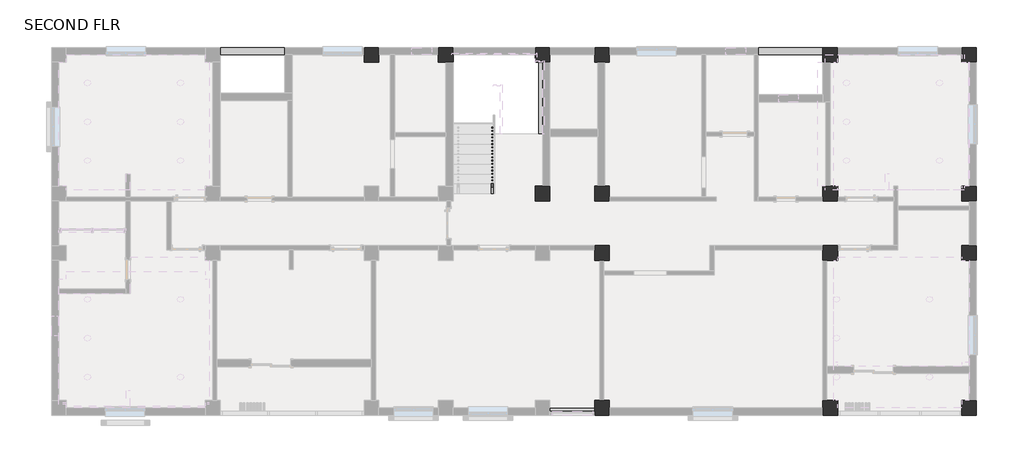
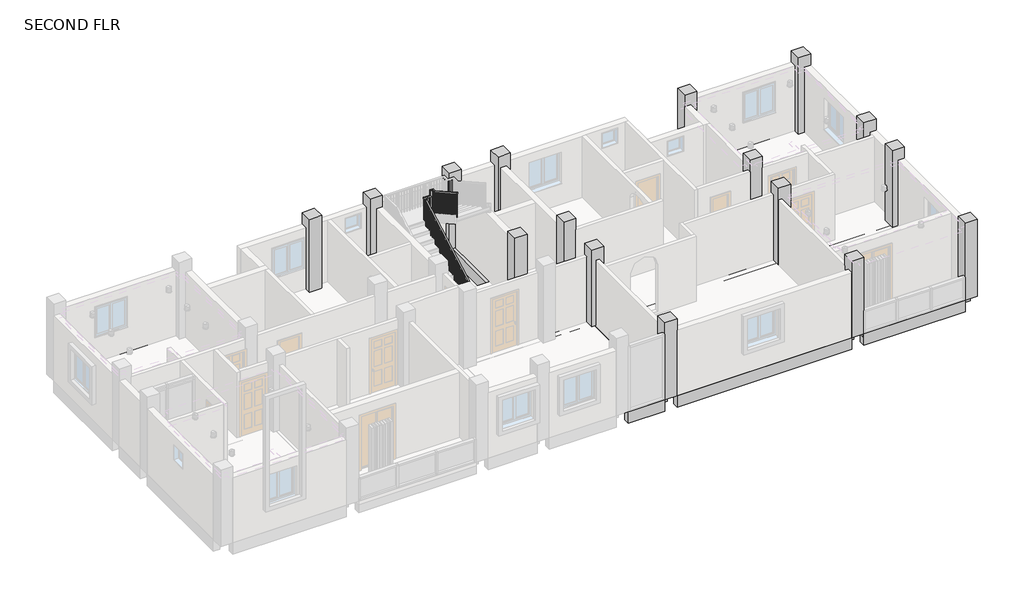
# One storey, part 4 of 5: 29 beams, 16 columns, 1 railing.
"""IFC4 building model written with IfcOpenShell, lengths in millimetres."""

from ifc_helpers import new_model, si_unit, frame, origin, place, context, project, spatial, polyline, outline, extrude, faceted_brep, element, save

model = new_model("IFC4")

# Units and contexts
model_context = context("Model", 3, world=origin())
ifc_project = project(units=[si_unit("LENGTHUNIT", "METRE", prefix="MILLI")], contexts=[model_context])

# Site, building, storey
site = spatial("IfcSite", under=ifc_project)
building = spatial("IfcBuilding", under=site)
storey = spatial("IfcBuildingStorey", under=building, Name="SECOND FLR", Elevation=6400.8)

# Beams
placement = place(None, origin())
element("IfcBeam", 1, ObjectType="Concrete-Rectangular Beam : 9\" X 18\" BEAM", at=placement, inside=storey, context=model_context, shape_type="SweptSolid", body=[
    extrude(outline(polyline([(1310.3916602, -10887.8679047), (1310.3916602, -11116.4679047), (-61.2083398, -11116.4679047), (-61.2083398, -10887.8679047), (1310.3916602, -10887.8679047)])), frame((0.0, 0.0, 5943.6), z_axis=(0.0, 0.0, 1.0), x_axis=(1.0, 0.0, 0.0)), (0.0, 0.0, 1.0), 457.2),
])
element("IfcBeam", 2, ObjectType="Concrete-Rectangular Beam : 9\" X 18\" BEAM", at=placement, inside=storey, context=model_context, shape_type="SweptSolid", body=[
    extrude(outline(polyline([(1424.6916602, -6358.3794704), (1653.2916602, -6358.3794704), (1653.2916602, -10659.2679047), (1424.6916602, -10659.2679047), (1424.6916602, -6358.3794704)])), frame((0.0, 0.0, 5943.6), z_axis=(0.0, 0.0, 1.0), x_axis=(1.0, 0.0, 0.0)), (0.0, 0.0, 1.0), 457.2),
])
element("IfcBeam", 3, ObjectType="Concrete-Rectangular Beam : 9\" X 18\" BEAM", at=placement, inside=storey, context=model_context, shape_type="SweptSolid", body=[
    extrude(outline(polyline([(1424.6916602, -4529.5794704), (1653.2916602, -4529.5794704), (1653.2916602, -5901.1794704), (1424.6916602, -5901.1794704), (1424.6916602, -4529.5794704)])), frame((0.0, 0.0, 5943.6), z_axis=(0.0, 0.0, 1.0), x_axis=(1.0, 0.0, 0.0)), (0.0, 0.0, 1.0), 457.2),
])
element("IfcBeam", 4, ObjectType="Concrete-Rectangular Beam : 9\" X 18\" BEAM", at=placement, inside=storey, context=model_context, shape_type="SweptSolid", body=[
    extrude(outline(polyline([(8317.2128058, -10887.8679047), (8317.2128058, -11116.4679047), (1767.5916602, -11116.4679047), (1767.5916602, -10887.8679047), (8317.2128058, -10887.8679047)])), frame((0.0, 0.0, 5943.6), z_axis=(0.0, 0.0, 1.0), x_axis=(1.0, 0.0, 0.0)), (0.0, 0.0, 1.0), 457.2),
])
element("IfcBeam", 5, ObjectType="Concrete-Rectangular Beam : 9\" X 18\" BEAM", at=placement, inside=storey, context=model_context, shape_type="SweptSolid", body=[
    extrude(outline(polyline([(12584.4128058, -10887.8679047), (12584.4128058, -11116.4679047), (8774.4128058, -11116.4679047), (8774.4128058, -10887.8679047), (12584.4128058, -10887.8679047)])), frame((0.0, 0.0, 5943.6), z_axis=(0.0, 0.0, 1.0), x_axis=(1.0, 0.0, 0.0)), (0.0, 0.0, 1.0), 457.2),
])
element("IfcBeam", 6, ObjectType="Concrete-Rectangular Beam : 9\" X 18\" BEAM", at=placement, inside=storey, context=model_context, shape_type="SweptSolid", body=[
    extrude(outline(polyline([(12813.0128058, -6358.3794704), (13041.6128058, -6358.3794704), (13041.6128058, -10659.2679047), (12813.0128058, -10659.2679047), (12813.0128058, -6358.3794704)])), frame((0.0, 0.0, 5943.6), z_axis=(0.0, 0.0, 1.0), x_axis=(1.0, 0.0, 0.0)), (0.0, 0.0, 1.0), 457.2),
])
element("IfcBeam", 7, ObjectType="Concrete-Rectangular Beam : 9\" X 18\" BEAM", at=placement, inside=storey, context=model_context, shape_type="SweptSolid", body=[
    extrude(outline(polyline([(12813.0128058, -4529.5794704), (13041.6128058, -4529.5794704), (13041.6128058, -5901.1794704), (12813.0128058, -5901.1794704), (12813.0128058, -4529.5794704)])), frame((0.0, 0.0, 5943.6), z_axis=(0.0, 0.0, 1.0), x_axis=(1.0, 0.0, 0.0)), (0.0, 0.0, 1.0), 457.2),
])
element("IfcBeam", 8, ObjectType="Concrete-Rectangular Beam : 9\" X 18\" BEAM", at=placement, inside=storey, context=model_context, shape_type="SweptSolid", body=[
    extrude(outline(polyline([(12813.0128058, -262.3794704), (13041.6128058, -262.3794704), (13041.6128058, -4072.3794704), (12813.0128058, -4072.3794704), (12813.0128058, -262.3794704)])), frame((0.0, 0.0, 5943.6), z_axis=(0.0, 0.0, 1.0), x_axis=(1.0, 0.0, 0.0)), (0.0, 0.0, 1.0), 457.2),
])
element("IfcBeam", 9, ObjectType="Concrete-Rectangular Beam : 9\" X 18\" BEAM", at=placement, inside=storey, context=model_context, shape_type="SweptSolid", body=[
    extrude(outline(polyline([(8774.4128058, -33.7794704), (8774.4128058, 194.8205296), (12584.4128058, 194.8205296), (12584.4128058, -33.7794704), (8774.4128058, -33.7794704)])), frame((0.0, 0.0, 5943.6), z_axis=(0.0, 0.0, 1.0), x_axis=(1.0, 0.0, 0.0)), (0.0, 0.0, 1.0), 457.2),
])
element("IfcBeam", 10, ObjectType="Concrete-Rectangular Beam : 9\" X 18\" BEAM", at=placement, inside=storey, context=model_context, shape_type="SweptSolid", body=[
    extrude(outline(polyline([(1767.5916602, -33.7794704), (1767.5916602, 194.8205296), (8317.2128058, 194.8205296), (8317.2128058, -33.7794704), (1767.5916602, -33.7794704)])), frame((0.0, 0.0, 5943.6), z_axis=(0.0, 0.0, 1.0), x_axis=(1.0, 0.0, 0.0)), (0.0, 0.0, 1.0), 457.2),
])
element("IfcBeam", 11, ObjectType="Concrete-Rectangular Beam : 9\" X 18\" BEAM", at=placement, inside=storey, context=model_context, shape_type="SweptSolid", body=[
    extrude(outline(polyline([(-61.2083398, -33.7794704), (-61.2083398, 194.8205296), (1310.3916602, 194.8205296), (1310.3916602, -33.7794704), (-61.2083398, -33.7794704)])), frame((0.0, 0.0, 5943.6), z_axis=(0.0, 0.0, 1.0), x_axis=(1.0, 0.0, 0.0)), (0.0, 0.0, 1.0), 457.2),
])
element("IfcBeam", 12, ObjectType="Concrete-Rectangular Beam : 9\" X 18\" BEAM", at=placement, inside=storey, context=model_context, shape_type="SweptSolid", body=[
    extrude(outline(polyline([(-3029.5456086, -33.7794704), (-3029.5456086, 194.8205296), (-518.4083398, 194.8205296), (-518.4083398, -33.7794704), (-3029.5456086, -33.7794704)])), frame((0.0, 0.0, 5943.6), z_axis=(0.0, 0.0, 1.0), x_axis=(1.0, 0.0, 0.0)), (0.0, 0.0, 1.0), 457.2),
])
element("IfcBeam", 13, ObjectType="Concrete-Rectangular Beam : 9\" X 18\" BEAM", at=placement, inside=storey, context=model_context, shape_type="SweptSolid", body=[
    extrude(outline(polyline([(-5315.5456086, -33.7794704), (-5315.5456086, 194.8205296), (-3486.7456086, 194.8205296), (-3486.7456086, -33.7794704), (-5315.5456086, -33.7794704)])), frame((0.0, 0.0, 5943.6), z_axis=(0.0, 0.0, 1.0), x_axis=(1.0, 0.0, 0.0)), (0.0, 0.0, 1.0), 457.2),
])
element("IfcBeam", 14, ObjectType="Concrete-Rectangular Beam : 9\" X 18\" BEAM", at=placement, inside=storey, context=model_context, shape_type="SweptSolid", body=[
    extrude(outline(polyline([(-10192.3456086, -33.7794704), (-10192.3456086, 194.8205296), (-5772.7456086, 194.8205296), (-5772.7456086, -33.7794704), (-10192.3456086, -33.7794704)])), frame((0.0, 0.0, 5943.6), z_axis=(0.0, 0.0, 1.0), x_axis=(1.0, 0.0, 0.0)), (0.0, 0.0, 1.0), 457.2),
])
element("IfcBeam", 15, ObjectType="Concrete-Rectangular Beam : 9\" X 18\" BEAM", at=placement, inside=storey, context=model_context, shape_type="SweptSolid", body=[
    extrude(outline(polyline([(-14916.7456086, -33.7794704), (-14916.7456086, 194.8205296), (-10649.5456086, 194.8205296), (-10649.5456086, -33.7794704), (-14916.7456086, -33.7794704)])), frame((0.0, 0.0, 5943.6), z_axis=(0.0, 0.0, 1.0), x_axis=(1.0, 0.0, 0.0)), (0.0, 0.0, 1.0), 457.2),
])
element("IfcBeam", 16, ObjectType="Concrete-Rectangular Beam : 9\" X 18\" BEAM", at=placement, inside=storey, context=model_context, shape_type="SweptSolid", body=[
    extrude(outline(polyline([(-518.4083398, -4186.6794704), (-518.4083398, -4415.2794704), (-3029.5456086, -4415.2794704), (-3029.5456086, -4186.6794704), (-518.4083398, -4186.6794704)])), frame((0.0, 0.0, 5943.6), z_axis=(0.0, 0.0, 1.0), x_axis=(1.0, 0.0, 0.0)), (0.0, 0.0, 1.0), 457.2),
])
element("IfcBeam", 17, ObjectType="Concrete-Rectangular Beam : 9\" X 18\" BEAM", at=placement, inside=storey, context=model_context, shape_type="SweptSolid", body=[
    extrude(outline(polyline([(1310.3916602, -4186.6794704), (1310.3916602, -4415.2794704), (-61.2083398, -4415.2794704), (-61.2083398, -4186.6794704), (1310.3916602, -4186.6794704)])), frame((0.0, 0.0, 5943.6), z_axis=(0.0, 0.0, 1.0), x_axis=(1.0, 0.0, 0.0)), (0.0, 0.0, 1.0), 457.2),
])
element("IfcBeam", 18, ObjectType="Concrete-Rectangular Beam : 9\" X 18\" BEAM", at=placement, inside=storey, context=model_context, shape_type="SweptSolid", body=[
    extrude(outline(polyline([(1424.6916602, -262.3794704), (1653.2916602, -262.3794704), (1653.2916602, -4072.3794704), (1424.6916602, -4072.3794704), (1424.6916602, -262.3794704)])), frame((0.0, 0.0, 5943.6), z_axis=(0.0, 0.0, 1.0), x_axis=(1.0, 0.0, 0.0)), (0.0, 0.0, 1.0), 457.2),
])
element("IfcBeam", 19, ObjectType="Concrete-Rectangular Beam : 9\" X 18\" BEAM", at=placement, inside=storey, context=model_context, shape_type="SweptSolid", body=[
    extrude(outline(polyline([(-175.5083398, -4072.3794704), (-404.1083398, -4072.3794704), (-404.1083398, -262.3794704), (-175.5083398, -262.3794704), (-175.5083398, -4072.3794704)])), frame((0.0, 0.0, 5943.6), z_axis=(0.0, 0.0, 1.0), x_axis=(1.0, 0.0, 0.0)), (0.0, 0.0, 1.0), 457.2),
])
element("IfcBeam", 20, ObjectType="Concrete-Rectangular Beam : 9\" X 18\" BEAM", at=placement, inside=storey, context=model_context, shape_type="SweptSolid", body=[
    extrude(outline(polyline([(-3143.8456086, -4072.3794704), (-3372.4456086, -4072.3794704), (-3372.4456086, -262.3794704), (-3143.8456086, -262.3794704), (-3143.8456086, -4072.3794704)])), frame((0.0, 0.0, 5943.6), z_axis=(0.0, 0.0, 1.0), x_axis=(1.0, 0.0, 0.0)), (0.0, 0.0, 1.0), 457.2),
])
element("IfcBeam", 21, ObjectType="Concrete-Rectangular Beam : 9\" X 18\" BEAM", at=placement, inside=storey, context=model_context, shape_type="SweptSolid", body=[
    extrude(outline(polyline([(-5429.8456086, -4072.3794704), (-5658.4456086, -4072.3794704), (-5658.4456086, -262.3794704), (-5429.8456086, -262.3794704), (-5429.8456086, -4072.3794704)])), frame((0.0, 0.0, 5943.6), z_axis=(0.0, 0.0, 1.0), x_axis=(1.0, 0.0, 0.0)), (0.0, 0.0, 1.0), 457.2),
])
element("IfcBeam", 22, ObjectType="Concrete-Rectangular Beam : 9\" X 18\" BEAM", at=placement, inside=storey, context=model_context, shape_type="SweptSolid", body=[
    extrude(outline(polyline([(1310.3916602, -6015.4794704), (1310.3916602, -6244.0794704), (-61.2083398, -6244.0794704), (-61.2083398, -6015.4794704), (1310.3916602, -6015.4794704)])), frame((0.0, 0.0, 5943.6), z_axis=(0.0, 0.0, 1.0), x_axis=(1.0, 0.0, 0.0)), (0.0, 0.0, 1.0), 457.2),
])
element("IfcBeam", 23, ObjectType="Concrete-Rectangular Beam : 9\" X 18\" BEAM", at=placement, inside=storey, context=model_context, shape_type="SweptSolid", body=[
    extrude(outline(polyline([(8317.2128058, -4186.6794704), (8317.2128058, -4415.2794704), (1767.5916602, -4415.2794704), (1767.5916602, -4186.6794704), (8317.2128058, -4186.6794704)])), frame((0.0, 0.0, 5943.6), z_axis=(0.0, 0.0, 1.0), x_axis=(1.0, 0.0, 0.0)), (0.0, 0.0, 1.0), 457.2),
])
element("IfcBeam", 24, ObjectType="Concrete-Rectangular Beam : 9\" X 18\" BEAM", at=placement, inside=storey, context=model_context, shape_type="SweptSolid", body=[
    extrude(outline(polyline([(12584.4128058, -4186.6794704), (12584.4128058, -4415.2794704), (8774.4128058, -4415.2794704), (8774.4128058, -4186.6794704), (12584.4128058, -4186.6794704)])), frame((0.0, 0.0, 5943.6), z_axis=(0.0, 0.0, 1.0), x_axis=(1.0, 0.0, 0.0)), (0.0, 0.0, 1.0), 457.2),
])
element("IfcBeam", 25, ObjectType="Concrete-Rectangular Beam : 9\" X 18\" BEAM", at=placement, inside=storey, context=model_context, shape_type="SweptSolid", body=[
    extrude(outline(polyline([(8774.4128058, -6244.0794704), (8774.4128058, -6015.4794704), (12584.4128058, -6015.4794704), (12584.4128058, -6244.0794704), (8774.4128058, -6244.0794704)])), frame((0.0, 0.0, 5943.6), z_axis=(0.0, 0.0, 1.0), x_axis=(1.0, 0.0, 0.0)), (0.0, 0.0, 1.0), 457.2),
])
element("IfcBeam", 26, ObjectType="Concrete-Rectangular Beam : 9\" X 18\" BEAM", at=placement, inside=storey, context=model_context, shape_type="SweptSolid", body=[
    extrude(outline(polyline([(1767.5916602, -6244.0794704), (1767.5916602, -6015.4794704), (8317.2128058, -6015.4794704), (8317.2128058, -6244.0794704), (1767.5916602, -6244.0794704)])), frame((0.0, 0.0, 5943.6), z_axis=(0.0, 0.0, 1.0), x_axis=(1.0, 0.0, 0.0)), (0.0, 0.0, 1.0), 457.2),
])
element("IfcBeam", 27, ObjectType="Concrete-Rectangular Beam : 9\" X 18\" BEAM", at=placement, inside=storey, context=model_context, shape_type="SweptSolid", body=[
    extrude(outline(polyline([(8431.5128058, -6358.3794704), (8660.1128058, -6358.3794704), (8660.1128058, -10659.2679047), (8431.5128058, -10659.2679047), (8431.5128058, -6358.3794704)])), frame((0.0, 0.0, 5943.6), z_axis=(0.0, 0.0, 1.0), x_axis=(1.0, 0.0, 0.0)), (0.0, 0.0, 1.0), 457.2),
])
element("IfcBeam", 28, ObjectType="Concrete-Rectangular Beam : 9\" X 18\" BEAM", at=placement, inside=storey, context=model_context, shape_type="SweptSolid", body=[
    extrude(outline(polyline([(8431.5128058, -4529.5794704), (8660.1128058, -4529.5794704), (8660.1128058, -5901.1794704), (8431.5128058, -5901.1794704), (8431.5128058, -4529.5794704)])), frame((0.0, 0.0, 5943.6), z_axis=(0.0, 0.0, 1.0), x_axis=(1.0, 0.0, 0.0)), (0.0, 0.0, 1.0), 457.2),
])
element("IfcBeam", 29, ObjectType="Concrete-Rectangular Beam : 9\" X 18\" BEAM", at=placement, inside=storey, context=model_context, shape_type="SweptSolid", body=[
    extrude(outline(polyline([(8431.5128058, -262.3794704), (8660.1128058, -262.3794704), (8660.1128058, -4072.3794704), (8431.5128058, -4072.3794704), (8431.5128058, -262.3794704)])), frame((0.0, 0.0, 5943.6), z_axis=(0.0, 0.0, 1.0), x_axis=(1.0, 0.0, 0.0)), (0.0, 0.0, 1.0), 457.2),
])

# Columns
element("IfcColumn", 30, ObjectType="Concrete-Rectangular-Column : COLUMN 18\" X 18\"", at=placement, inside=storey, context=model_context, shape_type="SweptSolid", body=[
    extrude(outline(polyline([(-5315.5456086, 194.8205296), (-5315.5456086, -262.3794704), (-5772.7456086, -262.3794704), (-5772.7456086, 194.8205296), (-5315.5456086, 194.8205296)])), frame((0.0, 0.0, 6400.8), z_axis=(0.0, 0.0, 1.0), x_axis=(1.0, 0.0, 0.0)), (0.0, 0.0, 1.0), 3048.0),
])
element("IfcColumn", 31, ObjectType="Concrete-Rectangular-Column : COLUMN 18\" X 18\"", at=placement, inside=storey, context=model_context, shape_type="SweptSolid", body=[
    extrude(outline(polyline([(-3029.5456086, 194.8205296), (-3029.5456086, -262.3794704), (-3486.7456086, -262.3794704), (-3486.7456086, 194.8205296), (-3029.5456086, 194.8205296)])), frame((0.0, 0.0, 6400.8), z_axis=(0.0, 0.0, 1.0), x_axis=(1.0, 0.0, 0.0)), (0.0, 0.0, 1.0), 3048.0),
])
element("IfcColumn", 32, ObjectType="Concrete-Rectangular-Column : COLUMN 18\" X 18\"", at=placement, inside=storey, context=model_context, shape_type="SweptSolid", body=[
    extrude(outline(polyline([(-61.2083398, 194.8205296), (-61.2083398, -262.3794704), (-518.4083398, -262.3794704), (-518.4083398, 194.8205296), (-61.2083398, 194.8205296)])), frame((0.0, 0.0, 6400.8), z_axis=(0.0, 0.0, 1.0), x_axis=(1.0, 0.0, 0.0)), (0.0, 0.0, 1.0), 3048.0),
])
element("IfcColumn", 33, ObjectType="Concrete-Rectangular-Column : COLUMN 18\" X 18\"", at=placement, inside=storey, context=model_context, shape_type="SweptSolid", body=[
    extrude(outline(polyline([(1767.5916602, 194.8205296), (1767.5916602, -262.3794704), (1310.3916602, -262.3794704), (1310.3916602, 194.8205296), (1767.5916602, 194.8205296)])), frame((0.0, 0.0, 6400.8), z_axis=(0.0, 0.0, 1.0), x_axis=(1.0, 0.0, 0.0)), (0.0, 0.0, 1.0), 3048.0),
])
element("IfcColumn", 34, ObjectType="Concrete-Rectangular-Column : COLUMN 18\" X 18\"", at=placement, inside=storey, context=model_context, shape_type="SweptSolid", body=[
    extrude(outline(polyline([(8774.4128058, 194.8205296), (8774.4128058, -262.3794704), (8317.2128058, -262.3794704), (8317.2128058, 194.8205296), (8774.4128058, 194.8205296)])), frame((0.0, 0.0, 6400.8), z_axis=(0.0, 0.0, 1.0), x_axis=(1.0, 0.0, 0.0)), (0.0, 0.0, 1.0), 3048.0),
])
element("IfcColumn", 35, ObjectType="Concrete-Rectangular-Column : COLUMN 18\" X 18\"", at=placement, inside=storey, context=model_context, shape_type="SweptSolid", body=[
    extrude(outline(polyline([(13041.6128058, 194.8205296), (13041.6128058, -262.3794704), (12584.4128058, -262.3794704), (12584.4128058, 194.8205296), (13041.6128058, 194.8205296)])), frame((0.0, 0.0, 6400.8), z_axis=(0.0, 0.0, 1.0), x_axis=(1.0, 0.0, 0.0)), (0.0, 0.0, 1.0), 3048.0),
])
element("IfcColumn", 36, ObjectType="Concrete-Rectangular-Column : COLUMN 18\" X 18\"", at=placement, inside=storey, context=model_context, shape_type="SweptSolid", body=[
    extrude(outline(polyline([(13041.6128058, -4072.3794704), (13041.6128058, -4529.5794704), (12584.4128058, -4529.5794704), (12584.4128058, -4072.3794704), (13041.6128058, -4072.3794704)])), frame((0.0, 0.0, 6400.8), z_axis=(0.0, 0.0, 1.0), x_axis=(1.0, 0.0, 0.0)), (0.0, 0.0, 1.0), 3048.0),
])
element("IfcColumn", 37, ObjectType="Concrete-Rectangular-Column : COLUMN 18\" X 18\"", at=placement, inside=storey, context=model_context, shape_type="SweptSolid", body=[
    extrude(outline(polyline([(13041.6128058, -5901.1794704), (13041.6128058, -6358.3794704), (12584.4128058, -6358.3794704), (12584.4128058, -5901.1794704), (13041.6128058, -5901.1794704)])), frame((0.0, 0.0, 6400.8), z_axis=(0.0, 0.0, 1.0), x_axis=(1.0, 0.0, 0.0)), (0.0, 0.0, 1.0), 3048.0),
])
element("IfcColumn", 38, ObjectType="Concrete-Rectangular-Column : COLUMN 18\" X 18\"", at=placement, inside=storey, context=model_context, shape_type="SweptSolid", body=[
    extrude(outline(polyline([(13041.6128058, -10659.2679047), (13041.6128058, -11116.4679047), (12584.4128058, -11116.4679047), (12584.4128058, -10659.2679047), (13041.6128058, -10659.2679047)])), frame((0.0, 0.0, 6400.8), z_axis=(0.0, 0.0, 1.0), x_axis=(1.0, 0.0, 0.0)), (0.0, 0.0, 1.0), 3048.0),
])
element("IfcColumn", 39, ObjectType="Concrete-Rectangular-Column : COLUMN 18\" X 18\"", at=placement, inside=storey, context=model_context, shape_type="SweptSolid", body=[
    extrude(outline(polyline([(8774.4128058, -10659.2679047), (8774.4128058, -11116.4679047), (8317.2128058, -11116.4679047), (8317.2128058, -10659.2679047), (8774.4128058, -10659.2679047)])), frame((0.0, 0.0, 6400.8), z_axis=(0.0, 0.0, 1.0), x_axis=(1.0, 0.0, 0.0)), (0.0, 0.0, 1.0), 3048.0),
])
element("IfcColumn", 40, ObjectType="Concrete-Rectangular-Column : COLUMN 18\" X 18\"", at=placement, inside=storey, context=model_context, shape_type="SweptSolid", body=[
    extrude(outline(polyline([(1767.5916602, -10659.2679047), (1767.5916602, -11116.4679047), (1310.3916602, -11116.4679047), (1310.3916602, -10659.2679047), (1767.5916602, -10659.2679047)])), frame((0.0, 0.0, 6400.8), z_axis=(0.0, 0.0, 1.0), x_axis=(1.0, 0.0, 0.0)), (0.0, 0.0, 1.0), 3048.0),
])
element("IfcColumn", 41, ObjectType="Concrete-Rectangular-Column : COLUMN 18\" X 18\"", at=placement, inside=storey, context=model_context, shape_type="SweptSolid", body=[
    extrude(outline(polyline([(-61.2083398, -4072.3794704), (-61.2083398, -4529.5794704), (-518.4083398, -4529.5794704), (-518.4083398, -4072.3794704), (-61.2083398, -4072.3794704)])), frame((0.0, 0.0, 6400.8), z_axis=(0.0, 0.0, 1.0), x_axis=(1.0, 0.0, 0.0)), (0.0, 0.0, 1.0), 3048.0),
])
element("IfcColumn", 42, ObjectType="Concrete-Rectangular-Column : COLUMN 18\" X 18\"", at=placement, inside=storey, context=model_context, shape_type="SweptSolid", body=[
    extrude(outline(polyline([(1767.5916602, -4072.3794704), (1767.5916602, -4529.5794704), (1310.3916602, -4529.5794704), (1310.3916602, -4072.3794704), (1767.5916602, -4072.3794704)])), frame((0.0, 0.0, 6400.8), z_axis=(0.0, 0.0, 1.0), x_axis=(1.0, 0.0, 0.0)), (0.0, 0.0, 1.0), 3048.0),
])
element("IfcColumn", 43, ObjectType="Concrete-Rectangular-Column : COLUMN 18\" X 18\"", at=placement, inside=storey, context=model_context, shape_type="SweptSolid", body=[
    extrude(outline(polyline([(8774.4128058, -4072.3794704), (8774.4128058, -4529.5794704), (8317.2128058, -4529.5794704), (8317.2128058, -4072.3794704), (8774.4128058, -4072.3794704)])), frame((0.0, 0.0, 6400.8), z_axis=(0.0, 0.0, 1.0), x_axis=(1.0, 0.0, 0.0)), (0.0, 0.0, 1.0), 3048.0),
])
element("IfcColumn", 44, ObjectType="Concrete-Rectangular-Column : COLUMN 18\" X 18\"", at=placement, inside=storey, context=model_context, shape_type="SweptSolid", body=[
    extrude(outline(polyline([(8774.4128058, -5901.1794704), (8774.4128058, -6358.3794704), (8317.2128058, -6358.3794704), (8317.2128058, -5901.1794704), (8774.4128058, -5901.1794704)])), frame((0.0, 0.0, 6400.8), z_axis=(0.0, 0.0, 1.0), x_axis=(1.0, 0.0, 0.0)), (0.0, 0.0, 1.0), 3048.0),
])
element("IfcColumn", 45, ObjectType="Concrete-Rectangular-Column : COLUMN 18\" X 18\"", at=placement, inside=storey, context=model_context, shape_type="SweptSolid", body=[
    extrude(outline(polyline([(1767.5916602, -5901.1794704), (1767.5916602, -6358.3794704), (1310.3916602, -6358.3794704), (1310.3916602, -5901.1794704), (1767.5916602, -5901.1794704)])), frame((0.0, 0.0, 6400.8), z_axis=(0.0, 0.0, 1.0), x_axis=(1.0, 0.0, 0.0)), (0.0, 0.0, 1.0), 3048.0),
])

# Railing
element("IfcRailing", 46, ObjectType="Handrail - Rectangular", at=placement, inside=storey, context=model_context, shape_type="SolidModel", body=[
    faceted_brep([(-1861.1456086, -4300.9794704, 7484.5333333), (-1861.1456086, -4300.9794704, 7426.420221), (-1810.3456086, -4300.9794704, 7426.420221), (-1810.3456086, -4300.9794704, 7484.5333333), (-1861.1456086, -1024.3794704, 9304.8666667), (-1861.1456086, -973.5794704, 9274.9757765), (-1810.3456086, -973.5794704, 9274.9757765), (-1810.3456086, -1024.3794704, 9304.8666667), (-1861.1456086, -1024.3794704, 9347.2), (-1861.1456086, -973.5794704, 9296.4), (-1810.3456086, -973.5794704, 9296.4), (-1810.3456086, -1024.3794704, 9347.2), (-1861.1456086, -897.3794704, 9347.2), (-1861.1456086, -897.3794704, 9296.4), (-1810.3456086, -948.1794704, 9296.4), (-1810.3456086, -948.1794704, 9347.2), (-1734.1456086, -897.3794704, 9347.2), (-1734.1456086, -897.3794704, 9296.4), (-1734.1456086, -948.1794704, 9296.4), (-1734.1456086, -948.1794704, 9347.2), (-1610.6083398, -897.3794704, 9347.2), (-1559.8083398, -897.3794704, 9296.4), (-1559.8083398, -948.1794704, 9296.4), (-1610.6083398, -948.1794704, 9347.2), (-1610.6083398, -897.3794704, 9558.8666667), (-1559.8083398, -897.3794704, 9508.0666667), (-1559.8083398, -948.1794704, 9508.0666667), (-1610.6083398, -948.1794704, 9558.8666667), (-1483.6083398, -897.3794704, 9558.8666667), (-1483.6083398, -897.3794704, 9508.0666667), (-1534.4083398, -948.1794704, 9508.0666667), (-1534.4083398, -948.1794704, 9558.8666667), (-1483.6083398, -1024.3794704, 9558.8666667), (-1483.6083398, -1037.5430727, 9508.0666667), (-1534.4083398, -1037.5430727, 9508.0666667), (-1534.4083398, -1024.3794704, 9558.8666667), (-1483.6083398, -2472.1794704, 10363.2), (-1534.4083398, -2472.1794704, 10363.2), (-1534.4083398, -2472.1794704, 10305.0868876), (-1483.6083398, -2472.1794704, 10305.0868876)], [[[0, 1, 2, 3]], [[1, 0, 4, 5]], [[2, 1, 5, 6]], [[3, 2, 6, 7]], [[0, 3, 7, 4]], [[5, 4, 8, 9]], [[6, 5, 9, 10]], [[7, 6, 10, 11]], [[4, 7, 11, 8]], [[9, 8, 12, 13]], [[10, 9, 13, 14]], [[11, 10, 14, 15]], [[8, 11, 15, 12]], [[13, 12, 16, 17]], [[14, 13, 17, 18]], [[15, 14, 18, 19]], [[12, 15, 19, 16]], [[17, 16, 20, 21]], [[18, 17, 21, 22]], [[19, 18, 22, 23]], [[16, 19, 23, 20]], [[21, 20, 24, 25]], [[22, 21, 25, 26]], [[23, 22, 26, 27]], [[20, 23, 27, 24]], [[25, 24, 28, 29]], [[26, 25, 29, 30]], [[27, 26, 30, 31]], [[24, 27, 31, 28]], [[29, 28, 32, 33]], [[30, 29, 33, 34]], [[31, 30, 34, 35]], [[28, 31, 35, 32]], [[36, 37, 38, 39]], [[33, 32, 36, 39]], [[34, 33, 39, 38]], [[35, 34, 38, 37]], [[32, 35, 37, 36]]]),
    extrude(outline(polyline([(-2456.3044704, 10296.2674432), (-2437.2544704, 10285.6841099), (-2437.2544704, 9279.4666667), (-2456.3044704, 9279.4666667), (-2456.3044704, 10296.2674432)])), frame((-1518.5333398, 0.0, 0.0), z_axis=(1.0, 0.0, 0.0), x_axis=(0.0, 1.0, 0.0)), (0.0, 0.0, 1.0), 19.05),
    extrude(outline(polyline([(-2354.7044704, 10239.8229988), (-2335.6544704, 10229.2396654), (-2335.6544704, 9279.4666667), (-2354.7044704, 9279.4666667), (-2354.7044704, 10239.8229988)])), frame((-1518.5333398, 0.0, 0.0), z_axis=(1.0, 0.0, 0.0), x_axis=(0.0, 1.0, 0.0)), (0.0, 0.0, 1.0), 19.05),
    extrude(outline(polyline([(-2253.1044704, 10183.3785543), (-2234.0544704, 10172.795221), (-2234.0544704, 9279.4666667), (-2253.1044704, 9279.4666667), (-2253.1044704, 10183.3785543)])), frame((-1518.5333398, 0.0, 0.0), z_axis=(1.0, 0.0, 0.0), x_axis=(0.0, 1.0, 0.0)), (0.0, 0.0, 1.0), 19.05),
    extrude(outline(polyline([(-2151.5044704, 10126.9341099), (-2132.4544704, 10116.3507765), (-2132.4544704, 9110.1333333), (-2151.5044704, 9110.1333333), (-2151.5044704, 10126.9341099)])), frame((-1518.5333398, 0.0, 0.0), z_axis=(1.0, 0.0, 0.0), x_axis=(0.0, 1.0, 0.0)), (0.0, 0.0, 1.0), 19.05),
    extrude(outline(polyline([(-2049.9044704, 10070.4896654), (-2030.8544704, 10059.9063321), (-2030.8544704, 9110.1333333), (-2049.9044704, 9110.1333333), (-2049.9044704, 10070.4896654)])), frame((-1518.5333398, 0.0, 0.0), z_axis=(1.0, 0.0, 0.0), x_axis=(0.0, 1.0, 0.0)), (0.0, 0.0, 1.0), 19.05),
    extrude(outline(polyline([(-1948.3044704, 10014.045221), (-1929.2544704, 10003.4618876), (-1929.2544704, 9110.1333333), (-1948.3044704, 9110.1333333), (-1948.3044704, 10014.045221)])), frame((-1518.5333398, 0.0, 0.0), z_axis=(1.0, 0.0, 0.0), x_axis=(0.0, 1.0, 0.0)), (0.0, 0.0, 1.0), 19.05),
    extrude(outline(polyline([(-1846.7044704, 9957.6007765), (-1827.6544704, 9947.0174432), (-1827.6544704, 8940.8), (-1846.7044704, 8940.8), (-1846.7044704, 9957.6007765)])), frame((-1518.5333398, 0.0, 0.0), z_axis=(1.0, 0.0, 0.0), x_axis=(0.0, 1.0, 0.0)), (0.0, 0.0, 1.0), 19.05),
    extrude(outline(polyline([(-1745.1044704, 9901.1563321), (-1726.0544704, 9890.5729988), (-1726.0544704, 8940.8), (-1745.1044704, 8940.8), (-1745.1044704, 9901.1563321)])), frame((-1518.5333398, 0.0, 0.0), z_axis=(1.0, 0.0, 0.0), x_axis=(0.0, 1.0, 0.0)), (0.0, 0.0, 1.0), 19.05),
    extrude(outline(polyline([(-1643.5044704, 9844.7118876), (-1624.4544704, 9834.1285543), (-1624.4544704, 8940.8), (-1643.5044704, 8940.8), (-1643.5044704, 9844.7118876)])), frame((-1518.5333398, 0.0, 0.0), z_axis=(1.0, 0.0, 0.0), x_axis=(0.0, 1.0, 0.0)), (0.0, 0.0, 1.0), 19.05),
    extrude(outline(polyline([(-1541.9044704, 9788.2674432), (-1522.8544704, 9777.6841099), (-1522.8544704, 8771.4666667), (-1541.9044704, 8771.4666667), (-1541.9044704, 9788.2674432)])), frame((-1518.5333398, 0.0, 0.0), z_axis=(1.0, 0.0, 0.0), x_axis=(0.0, 1.0, 0.0)), (0.0, 0.0, 1.0), 19.05),
    extrude(outline(polyline([(-1440.3044704, 9731.8229988), (-1421.2544704, 9721.2396654), (-1421.2544704, 8771.4666667), (-1440.3044704, 8771.4666667), (-1440.3044704, 9731.8229988)])), frame((-1518.5333398, 0.0, 0.0), z_axis=(1.0, 0.0, 0.0), x_axis=(0.0, 1.0, 0.0)), (0.0, 0.0, 1.0), 19.05),
    extrude(outline(polyline([(-1338.7044704, 9675.3785543), (-1319.6544704, 9664.795221), (-1319.6544704, 8771.4666667), (-1338.7044704, 8771.4666667), (-1338.7044704, 9675.3785543)])), frame((-1518.5333398, 0.0, 0.0), z_axis=(1.0, 0.0, 0.0), x_axis=(0.0, 1.0, 0.0)), (0.0, 0.0, 1.0), 19.05),
    extrude(outline(polyline([(-1237.1044704, 9618.9341099), (-1218.0544704, 9608.3507765), (-1218.0544704, 8602.1333333), (-1237.1044704, 8602.1333333), (-1237.1044704, 9618.9341099)])), frame((-1518.5333398, 0.0, 0.0), z_axis=(1.0, 0.0, 0.0), x_axis=(0.0, 1.0, 0.0)), (0.0, 0.0, 1.0), 19.05),
    extrude(outline(polyline([(-1135.5044704, 9562.4896654), (-1116.4544704, 9551.9063321), (-1116.4544704, 8602.1333333), (-1135.5044704, 8602.1333333), (-1135.5044704, 9562.4896654)])), frame((-1518.5333398, 0.0, 0.0), z_axis=(1.0, 0.0, 0.0), x_axis=(0.0, 1.0, 0.0)), (0.0, 0.0, 1.0), 19.05),
    extrude(outline(polyline([(-1033.9044704, 9506.045221), (-1014.8544704, 9495.4618876), (-1014.8544704, 8602.1333333), (-1033.9044704, 8602.1333333), (-1033.9044704, 9506.045221)])), frame((-1518.5333398, 0.0, 0.0), z_axis=(1.0, 0.0, 0.0), x_axis=(0.0, 1.0, 0.0)), (0.0, 0.0, 1.0), 19.05),
    extrude(outline(polyline([(-1540.4706086, -932.3044704), (-1540.4706086, -913.2544704), (-1521.4206086, -913.2544704), (-1521.4206086, -932.3044704), (-1540.4706086, -932.3044704)])), frame((0.0, 0.0, 8432.8), z_axis=(0.0, 0.0, 1.0), x_axis=(1.0, 0.0, 0.0)), (0.0, 0.0, 1.0), 1075.2666667),
    extrude(outline(polyline([(-1642.0706086, -932.3044704), (-1642.0706086, -913.2544704), (-1623.0206086, -913.2544704), (-1623.0206086, -932.3044704), (-1642.0706086, -932.3044704)])), frame((0.0, 0.0, 8432.8), z_axis=(0.0, 0.0, 1.0), x_axis=(1.0, 0.0, 0.0)), (0.0, 0.0, 1.0), 863.6),
    extrude(outline(polyline([(-1743.6706086, -932.3044704), (-1743.6706086, -913.2544704), (-1724.6206086, -913.2544704), (-1724.6206086, -932.3044704), (-1743.6706086, -932.3044704)])), frame((0.0, 0.0, 8432.8), z_axis=(0.0, 0.0, 1.0), x_axis=(1.0, 0.0, 0.0)), (0.0, 0.0, 1.0), 863.6),
    extrude(outline(polyline([(-1826.2206086, -957.7044704), (-1845.2706086, -957.7044704), (-1845.2706086, -938.6544704), (-1826.2206086, -938.6544704), (-1826.2206086, -957.7044704)])), frame((0.0, 0.0, 8432.8), z_axis=(0.0, 0.0, 1.0), x_axis=(1.0, 0.0, 0.0)), (0.0, 0.0, 1.0), 863.6),
    extrude(outline(polyline([(-1059.3044704, 9227.3507765), (-1040.2544704, 9237.9341099), (-1040.2544704, 8263.4666667), (-1059.3044704, 8263.4666667), (-1059.3044704, 9227.3507765)])), frame((-1845.2706086, 0.0, 0.0), z_axis=(1.0, 0.0, 0.0), x_axis=(0.0, 1.0, 0.0)), (0.0, 0.0, 1.0), 19.05),
    extrude(outline(polyline([(-1160.9044704, 9170.9063321), (-1141.8544704, 9181.4896654), (-1141.8544704, 8263.4666667), (-1160.9044704, 8263.4666667), (-1160.9044704, 9170.9063321)])), frame((-1845.2706086, 0.0, 0.0), z_axis=(1.0, 0.0, 0.0), x_axis=(0.0, 1.0, 0.0)), (0.0, 0.0, 1.0), 19.05),
    extrude(outline(polyline([(-1262.5044704, 9114.4618876), (-1243.4544704, 9125.045221), (-1243.4544704, 8263.4666667), (-1262.5044704, 8263.4666667), (-1262.5044704, 9114.4618876)])), frame((-1845.2706086, 0.0, 0.0), z_axis=(1.0, 0.0, 0.0), x_axis=(0.0, 1.0, 0.0)), (0.0, 0.0, 1.0), 19.05),
    extrude(outline(polyline([(-1364.1044704, 9058.0174432), (-1345.0544704, 9068.6007765), (-1345.0544704, 8094.1333333), (-1364.1044704, 8094.1333333), (-1364.1044704, 9058.0174432)])), frame((-1845.2706086, 0.0, 0.0), z_axis=(1.0, 0.0, 0.0), x_axis=(0.0, 1.0, 0.0)), (0.0, 0.0, 1.0), 19.05),
    extrude(outline(polyline([(-1465.7044704, 9001.5729988), (-1446.6544704, 9012.1563321), (-1446.6544704, 8094.1333333), (-1465.7044704, 8094.1333333), (-1465.7044704, 9001.5729988)])), frame((-1845.2706086, 0.0, 0.0), z_axis=(1.0, 0.0, 0.0), x_axis=(0.0, 1.0, 0.0)), (0.0, 0.0, 1.0), 19.05),
    extrude(outline(polyline([(-1567.3044704, 8945.1285543), (-1548.2544704, 8955.7118876), (-1548.2544704, 8094.1333333), (-1567.3044704, 8094.1333333), (-1567.3044704, 8945.1285543)])), frame((-1845.2706086, 0.0, 0.0), z_axis=(1.0, 0.0, 0.0), x_axis=(0.0, 1.0, 0.0)), (0.0, 0.0, 1.0), 19.05),
    extrude(outline(polyline([(-1668.9044704, 8888.6841099), (-1649.8544704, 8899.2674432), (-1649.8544704, 7924.8), (-1668.9044704, 7924.8), (-1668.9044704, 8888.6841099)])), frame((-1845.2706086, 0.0, 0.0), z_axis=(1.0, 0.0, 0.0), x_axis=(0.0, 1.0, 0.0)), (0.0, 0.0, 1.0), 19.05),
    extrude(outline(polyline([(-1770.5044704, 8832.2396654), (-1751.4544704, 8842.8229988), (-1751.4544704, 7924.8), (-1770.5044704, 7924.8), (-1770.5044704, 8832.2396654)])), frame((-1845.2706086, 0.0, 0.0), z_axis=(1.0, 0.0, 0.0), x_axis=(0.0, 1.0, 0.0)), (0.0, 0.0, 1.0), 19.05),
    extrude(outline(polyline([(-1872.1044704, 8775.795221), (-1853.0544704, 8786.3785543), (-1853.0544704, 7924.8), (-1872.1044704, 7924.8), (-1872.1044704, 8775.795221)])), frame((-1845.2706086, 0.0, 0.0), z_axis=(1.0, 0.0, 0.0), x_axis=(0.0, 1.0, 0.0)), (0.0, 0.0, 1.0), 19.05),
    extrude(outline(polyline([(-1973.7044704, 8719.3507765), (-1954.6544704, 8729.9341099), (-1954.6544704, 7755.4666667), (-1973.7044704, 7755.4666667), (-1973.7044704, 8719.3507765)])), frame((-1845.2706086, 0.0, 0.0), z_axis=(1.0, 0.0, 0.0), x_axis=(0.0, 1.0, 0.0)), (0.0, 0.0, 1.0), 19.05),
    extrude(outline(polyline([(-2075.3044704, 8662.9063321), (-2056.2544704, 8673.4896654), (-2056.2544704, 7755.4666667), (-2075.3044704, 7755.4666667), (-2075.3044704, 8662.9063321)])), frame((-1845.2706086, 0.0, 0.0), z_axis=(1.0, 0.0, 0.0), x_axis=(0.0, 1.0, 0.0)), (0.0, 0.0, 1.0), 19.05),
    extrude(outline(polyline([(-2176.9044704, 8606.4618876), (-2157.8544704, 8617.045221), (-2157.8544704, 7755.4666667), (-2176.9044704, 7755.4666667), (-2176.9044704, 8606.4618876)])), frame((-1845.2706086, 0.0, 0.0), z_axis=(1.0, 0.0, 0.0), x_axis=(0.0, 1.0, 0.0)), (0.0, 0.0, 1.0), 19.05),
    extrude(outline(polyline([(-2278.5044704, 8550.0174432), (-2259.4544704, 8560.6007765), (-2259.4544704, 7586.1333333), (-2278.5044704, 7586.1333333), (-2278.5044704, 8550.0174432)])), frame((-1845.2706086, 0.0, 0.0), z_axis=(1.0, 0.0, 0.0), x_axis=(0.0, 1.0, 0.0)), (0.0, 0.0, 1.0), 19.05),
    extrude(outline(polyline([(-2380.1044704, 8493.5729988), (-2361.0544704, 8504.1563321), (-2361.0544704, 7586.1333333), (-2380.1044704, 7586.1333333), (-2380.1044704, 8493.5729988)])), frame((-1845.2706086, 0.0, 0.0), z_axis=(1.0, 0.0, 0.0), x_axis=(0.0, 1.0, 0.0)), (0.0, 0.0, 1.0), 19.05),
    extrude(outline(polyline([(-2481.7044704, 8437.1285543), (-2462.6544704, 8447.7118876), (-2462.6544704, 7586.1333333), (-2481.7044704, 7586.1333333), (-2481.7044704, 8437.1285543)])), frame((-1845.2706086, 0.0, 0.0), z_axis=(1.0, 0.0, 0.0), x_axis=(0.0, 1.0, 0.0)), (0.0, 0.0, 1.0), 19.05),
    extrude(outline(polyline([(-2583.3044704, 8380.6841099), (-2564.2544704, 8391.2674432), (-2564.2544704, 7416.8), (-2583.3044704, 7416.8), (-2583.3044704, 8380.6841099)])), frame((-1845.2706086, 0.0, 0.0), z_axis=(1.0, 0.0, 0.0), x_axis=(0.0, 1.0, 0.0)), (0.0, 0.0, 1.0), 19.05),
    extrude(outline(polyline([(-2684.9044704, 8324.2396654), (-2665.8544704, 8334.8229988), (-2665.8544704, 7416.8), (-2684.9044704, 7416.8), (-2684.9044704, 8324.2396654)])), frame((-1845.2706086, 0.0, 0.0), z_axis=(1.0, 0.0, 0.0), x_axis=(0.0, 1.0, 0.0)), (0.0, 0.0, 1.0), 19.05),
    extrude(outline(polyline([(-2786.5044704, 8267.795221), (-2767.4544704, 8278.3785543), (-2767.4544704, 7416.8), (-2786.5044704, 7416.8), (-2786.5044704, 8267.795221)])), frame((-1845.2706086, 0.0, 0.0), z_axis=(1.0, 0.0, 0.0), x_axis=(0.0, 1.0, 0.0)), (0.0, 0.0, 1.0), 19.05),
    extrude(outline(polyline([(-2888.1044704, 8211.3507765), (-2869.0544704, 8221.9341099), (-2869.0544704, 7247.4666667), (-2888.1044704, 7247.4666667), (-2888.1044704, 8211.3507765)])), frame((-1845.2706086, 0.0, 0.0), z_axis=(1.0, 0.0, 0.0), x_axis=(0.0, 1.0, 0.0)), (0.0, 0.0, 1.0), 19.05),
    extrude(outline(polyline([(-2989.7044704, 8154.9063321), (-2970.6544704, 8165.4896654), (-2970.6544704, 7247.4666667), (-2989.7044704, 7247.4666667), (-2989.7044704, 8154.9063321)])), frame((-1845.2706086, 0.0, 0.0), z_axis=(1.0, 0.0, 0.0), x_axis=(0.0, 1.0, 0.0)), (0.0, 0.0, 1.0), 19.05),
    extrude(outline(polyline([(-3091.3044704, 8098.4618876), (-3072.2544704, 8109.045221), (-3072.2544704, 7247.4666667), (-3091.3044704, 7247.4666667), (-3091.3044704, 8098.4618876)])), frame((-1845.2706086, 0.0, 0.0), z_axis=(1.0, 0.0, 0.0), x_axis=(0.0, 1.0, 0.0)), (0.0, 0.0, 1.0), 19.05),
    extrude(outline(polyline([(-3192.9044704, 8042.0174432), (-3173.8544704, 8052.6007765), (-3173.8544704, 7078.1333333), (-3192.9044704, 7078.1333333), (-3192.9044704, 8042.0174432)])), frame((-1845.2706086, 0.0, 0.0), z_axis=(1.0, 0.0, 0.0), x_axis=(0.0, 1.0, 0.0)), (0.0, 0.0, 1.0), 19.05),
    extrude(outline(polyline([(-3294.5044704, 7985.5729988), (-3275.4544704, 7996.1563321), (-3275.4544704, 7078.1333333), (-3294.5044704, 7078.1333333), (-3294.5044704, 7985.5729988)])), frame((-1845.2706086, 0.0, 0.0), z_axis=(1.0, 0.0, 0.0), x_axis=(0.0, 1.0, 0.0)), (0.0, 0.0, 1.0), 19.05),
    extrude(outline(polyline([(-3396.1044704, 7929.1285543), (-3377.0544704, 7939.7118876), (-3377.0544704, 7078.1333333), (-3396.1044704, 7078.1333333), (-3396.1044704, 7929.1285543)])), frame((-1845.2706086, 0.0, 0.0), z_axis=(1.0, 0.0, 0.0), x_axis=(0.0, 1.0, 0.0)), (0.0, 0.0, 1.0), 19.05),
    extrude(outline(polyline([(-3497.7044704, 7872.6841099), (-3478.6544704, 7883.2674432), (-3478.6544704, 6908.8), (-3497.7044704, 6908.8), (-3497.7044704, 7872.6841099)])), frame((-1845.2706086, 0.0, 0.0), z_axis=(1.0, 0.0, 0.0), x_axis=(0.0, 1.0, 0.0)), (0.0, 0.0, 1.0), 19.05),
    extrude(outline(polyline([(-3599.3044704, 7816.2396654), (-3580.2544704, 7826.8229988), (-3580.2544704, 6908.8), (-3599.3044704, 6908.8), (-3599.3044704, 7816.2396654)])), frame((-1845.2706086, 0.0, 0.0), z_axis=(1.0, 0.0, 0.0), x_axis=(0.0, 1.0, 0.0)), (0.0, 0.0, 1.0), 19.05),
    extrude(outline(polyline([(-3700.9044704, 7759.795221), (-3681.8544704, 7770.3785543), (-3681.8544704, 6908.8), (-3700.9044704, 6908.8), (-3700.9044704, 7759.795221)])), frame((-1845.2706086, 0.0, 0.0), z_axis=(1.0, 0.0, 0.0), x_axis=(0.0, 1.0, 0.0)), (0.0, 0.0, 1.0), 19.05),
    extrude(outline(polyline([(-3802.5044704, 7703.3507765), (-3783.4544704, 7713.9341099), (-3783.4544704, 6739.4666667), (-3802.5044704, 6739.4666667), (-3802.5044704, 7703.3507765)])), frame((-1845.2706086, 0.0, 0.0), z_axis=(1.0, 0.0, 0.0), x_axis=(0.0, 1.0, 0.0)), (0.0, 0.0, 1.0), 19.05),
    extrude(outline(polyline([(-3904.1044704, 7646.9063321), (-3885.0544704, 7657.4896654), (-3885.0544704, 6739.4666667), (-3904.1044704, 6739.4666667), (-3904.1044704, 7646.9063321)])), frame((-1845.2706086, 0.0, 0.0), z_axis=(1.0, 0.0, 0.0), x_axis=(0.0, 1.0, 0.0)), (0.0, 0.0, 1.0), 19.05),
    extrude(outline(polyline([(-4005.7044704, 7590.4618876), (-3986.6544704, 7601.045221), (-3986.6544704, 6739.4666667), (-4005.7044704, 6739.4666667), (-4005.7044704, 7590.4618876)])), frame((-1845.2706086, 0.0, 0.0), z_axis=(1.0, 0.0, 0.0), x_axis=(0.0, 1.0, 0.0)), (0.0, 0.0, 1.0), 19.05),
    extrude(outline(polyline([(-4107.3044704, 7534.0174432), (-4088.2544704, 7544.6007765), (-4088.2544704, 6570.1333333), (-4107.3044704, 6570.1333333), (-4107.3044704, 7534.0174432)])), frame((-1845.2706086, 0.0, 0.0), z_axis=(1.0, 0.0, 0.0), x_axis=(0.0, 1.0, 0.0)), (0.0, 0.0, 1.0), 19.05),
    extrude(outline(polyline([(-4208.9044704, 7477.5729988), (-4189.8544704, 7488.1563321), (-4189.8544704, 6570.1333333), (-4208.9044704, 6570.1333333), (-4208.9044704, 7477.5729988)])), frame((-1845.2706086, 0.0, 0.0), z_axis=(1.0, 0.0, 0.0), x_axis=(0.0, 1.0, 0.0)), (0.0, 0.0, 1.0), 19.05),
    extrude(outline(polyline([(-1518.5333398, -932.3044704), (-1518.5333398, -913.2544704), (-1499.4833398, -913.2544704), (-1499.4833398, -932.3044704), (-1518.5333398, -932.3044704)])), frame((0.0, 0.0, 8432.8), z_axis=(0.0, 0.0, 1.0), x_axis=(1.0, 0.0, 0.0)), (0.0, 0.0, 1.0), 1075.2666667),
    extrude(outline(polyline([(-1826.2206086, -932.3044704), (-1845.2706086, -932.3044704), (-1845.2706086, -913.2544704), (-1826.2206086, -913.2544704), (-1826.2206086, -932.3044704)])), frame((0.0, 0.0, 8432.8), z_axis=(0.0, 0.0, 1.0), x_axis=(1.0, 0.0, 0.0)), (0.0, 0.0, 1.0), 863.6),
    extrude(outline(polyline([(-2472.1794704, 10305.0868876), (-2453.1294704, 10294.5035543), (-2453.1294704, 9279.4666667), (-2472.1794704, 9279.4666667), (-2472.1794704, 10305.0868876)])), frame((-1518.5333398, 0.0, 0.0), z_axis=(1.0, 0.0, 0.0), x_axis=(0.0, 1.0, 0.0)), (0.0, 0.0, 1.0), 19.05),
    extrude(outline(polyline([(-4300.9794704, 7426.420221), (-4281.9294704, 7437.0035543), (-4281.9294704, 6570.1333333), (-4300.9794704, 6570.1333333), (-4300.9794704, 7426.420221)])), frame((-1845.2706086, 0.0, 0.0), z_axis=(1.0, 0.0, 0.0), x_axis=(0.0, 1.0, 0.0)), (0.0, 0.0, 1.0), 19.05),
])

save(model, "model.ifc")

# Revit data of these elements
# Type "Concrete-Rectangular Beam : 9\" X 18\" BEAM"
#   Assembly Code = "B10"
#   Length [instance default] = 5' - 0"
#   b = 0' - 9"
#   h = 1' - 6"
#   Structural Material [instance default] = Concrete, Cast-in-Place gray
# Type "Concrete-Rectangular-Column : COLUMN 18\" X 18\""
#   Assembly Code = "B10"
#   b = 1' - 6"
#   h = 1' - 6"
#   Structural Material [instance default] = Concrete, Cast-in-Place gray
# Type "Handrail - Rectangular"
#   Assembly Code = "C2010400"
#   built-in parameter 1008612 = 0.0416667 (stored number, unit not read)
#   built-in parameter 1008611 = 0.0416667 (stored number, unit not read)
#   built-in parameter 1008609 = 0.333333 (stored number, unit not read)
#   built-in parameter 1008604 = 0.166667 (stored number, unit not read)
#   built-in parameter 1008603 = 0.166667 (stored number, unit not read)
#   Railing Height = 3' - 0"
#   built-in parameter 1008630 = 2
#   built-in parameter 1008610 = 2
#   built-in parameter 1008618 = Baluster - Square : 3/4"
# Elements 1, 4, 5, 6, 7, 8, 9, 10, 11, 12, 13, 14, 15 (IfcBeam, "Concrete-Rectangular Beam : 9\" X 18\" BEAM")
#   Structural Material = Concrete, Cast-in-Place gray
#   Phase Created = New Construction
#   Materials on its faces: "Concrete, Cast-in-Place gray", "SAND BEIGE PAINT"
# Elements 2, 3, 16, 17, 18, 19, 20, 21, 22, 23, 24, 25, 26, 27, 28, 29 (IfcBeam, "Concrete-Rectangular Beam : 9\" X 18\" BEAM")
#   Structural Material = Concrete, Cast-in-Place gray
#   Phase Created = New Construction
#   Materials on its faces: "Concrete, Cast-in-Place gray"
# Elements 30, 31, 32, 33, 34, 35, 36, 37, 38, 39, 40 (IfcColumn, "Concrete-Rectangular-Column : COLUMN 18\" X 18\"")
#   Structural Material = Concrete, Cast-in-Place gray
#   Phase Created = New Construction
#   Materials on its faces: "Concrete, Cast-in-Place gray", "SAND BEIGE PAINT"
# Elements 41, 42, 43, 44, 45 (IfcColumn, "Concrete-Rectangular-Column : COLUMN 18\" X 18\"")
#   Structural Material = Concrete, Cast-in-Place gray
#   Phase Created = New Construction
#   Materials on its faces: "Concrete, Cast-in-Place gray"
# Element 46 (IfcRailing, "Handrail - Rectangular")
#   Phase Created = New Construction
# Materials
#   "Concrete, Cast-in-Place gray": class "Concrete", colour RGB 192 192 192, transparency 0, Description = "Cast-in-place concrete", Cost = 0
#   "SAND BEIGE PAINT": class "Generic", colour RGB 120 120 120, transparency 0, Cost = 0
